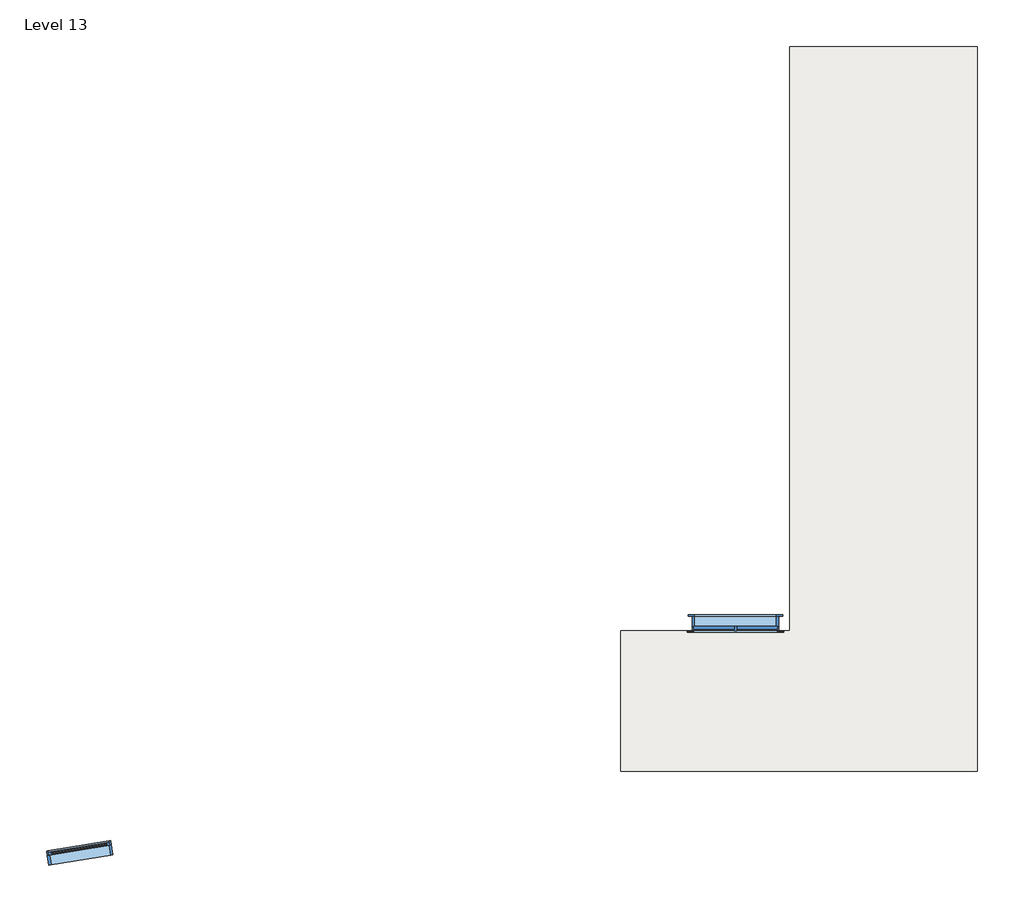
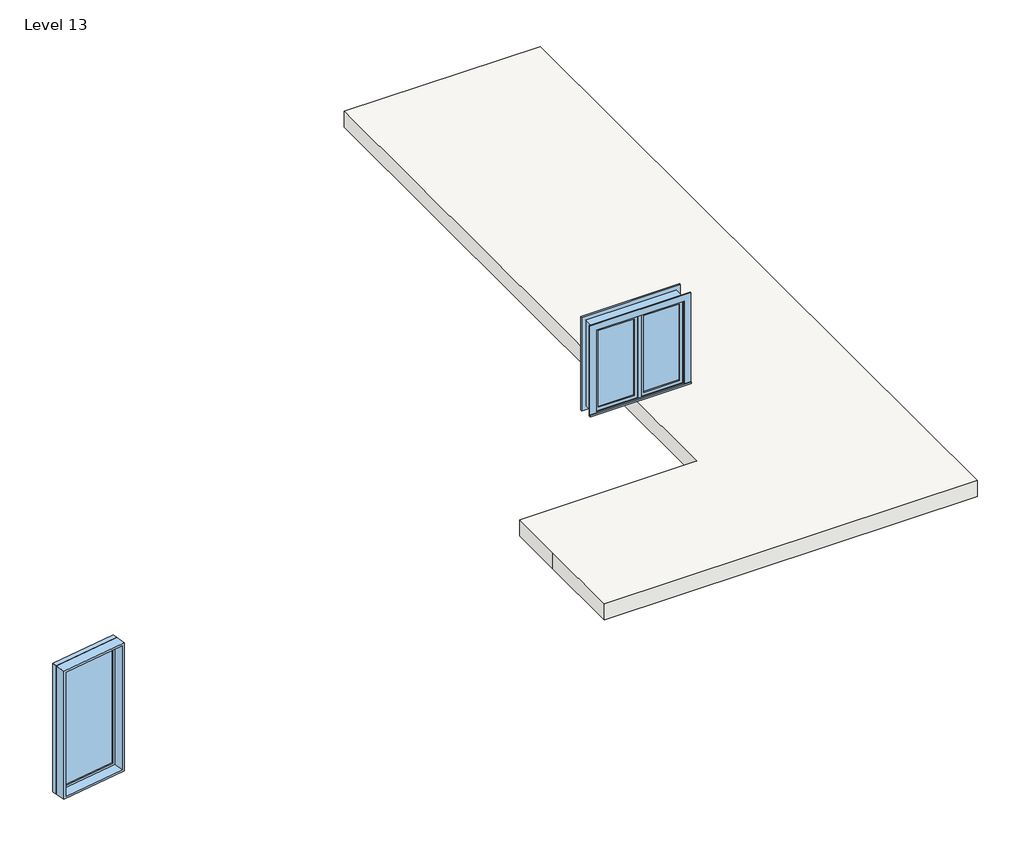
# One storey: 2 windows, 1 slab.
"""IFC4 building model written with IfcOpenShell, lengths in millimetres."""

from ifc_helpers import new_model, si_unit, frame, origin, place, context, project, spatial, polyline, outline, extrude, transform, mapped, element, save
from components import window_0862ab64, window_9a779fa2

model = new_model("IFC4")

# Units and contexts
model_context = context("Model", 3, world=origin())
ifc_project = project(units=[si_unit("LENGTHUNIT", "METRE", prefix="MILLI")], contexts=[model_context])

# Site, building, storey
site = spatial("IfcSite", under=ifc_project)
building = spatial("IfcBuilding", under=site)
storey = spatial("IfcBuildingStorey", under=building, Name="Level 13", Elevation=19659.6)

# Slab
placement = place(None, origin())
element("IfcSlab", 1, ObjectType="9\"", at=placement, inside=storey, context=model_context, shape_type="SweptSolid", body=[
    extrude(outline(polyline([(5039.2964723, -14840.0808221), (5039.2964723, -14078.0808221), (7223.6964723, -14078.0808221), (7426.8964723, -14078.0808221), (7426.8964723, -5848.4808221), (10068.4964723, -5848.4808221), (10068.4964723, -14840.0808221), (10068.4964723, -16059.2808221), (5039.2964723, -16059.2808221), (5039.2964723, -14840.0808221)])), frame((0.0, 0.0, 19431.0), z_axis=(0.0, 0.0, 1.0), x_axis=(1.0, 0.0, 0.0)), (0.0, 0.0, 1.0), 228.6),
])

# Windows
window_shape = window_0862ab64(model_context)
element("IfcWindow", 2, ObjectType="Casement Dbl with Trim : 48\" x 48\"", at=placement, inside=storey, context=model_context, shape_type="MappedRepresentation", body=[
    mapped(window_shape, transform((6658.4494573, -13957.4308221, 19899.9127534), x_axis=(-1.0, 0.0, 0.0), y_axis=(0.0, -1.0, 0.0), z_axis=(0.0, 0.0, 1.0))),
])
window_2_shape = window_9a779fa2(model_context)
element("IfcWindow", 3, ObjectType="Fixed : 36\" x 72\"", at=placement, inside=storey, context=model_context, shape_type="MappedRepresentation", body=[
    mapped(window_2_shape, transform((-2543.099786, -17204.6888165, 20190.5324703), x_axis=(0.9866375910039796, 0.16293024279692148, 0.0), y_axis=(-0.16293024279692148, 0.9866375910039796, 0.0), z_axis=(0.0, 0.0, 1.0))),
])

save(model, "model.ifc")

# Revit data of these elements
# Type "9\""
#   Assembly Code = "B1010"
#   Function = 0
#   Layers, outside or top first: 0' - 9" no material (function 1)
# Type "Casement Dbl with Trim : 48\" x 48\""
#   Type Mark = "10"
#   Construction Type Id = "GSP4R"
#   Assembly Code = "B2020100"
#   Analytic Construction = "1/8 in Pilkington single glazing"
#   Visual Light Transmittance = 0.9
#   Solar Heat Gain Coefficient = 0.78
#   Heat Transfer Coefficient (U) = 0.6496 BTU/(h·ft²·°F)
#   Height = 4' - 0"
#   Default Sill Height = 3' - 0"
#   Trim Projection - Ext. = 0' - 0 1/2"
#   Trim Projection - Int. = 0' - 0 3/4"
#   Trim Width - Exterior = 0' - 3 1/2"
#   Trim Width - Interior = 0' - 3 1/2"
#   Width = 4' - 0"
#   Window Inset = 0' - 0 3/4"
#   Define Thermal Properties by = 1
#   Glass Pane Material = Glass
#   Sash Material = Sash
#   Trim Exterior Material = Trim
#   Trim Interior Material = Trim
#   Wall Closure = (empty or 0)
# Type "Fixed : 36\" x 72\""
#   Type Mark = "9"
#   Construction Type Id = "GSP4R"
#   Assembly Code = "B2020100"
#   Analytic Construction = "1/8 in Pilkington single glazing"
#   Visual Light Transmittance = 0.9
#   Solar Heat Gain Coefficient = 0.78
#   Heat Transfer Coefficient (U) = 0.6496 BTU/(h·ft²·°F)
#   Height = 6' - 0"
#   Default Sill Height = 1' - 0"
#   Width = 3' - 0"
#   Window Inset = 0' - 0 3/4"
#   Define Thermal Properties by = 1
#   Glass Pane Material = Glass
#   Sash Material = Sash
#   Wall Closure = (empty or 0)
# Element 1 (IfcSlab, "9\"")
#   built-in parameter 1001955 = -1.5708 (stored number, unit not read)
#   Height Offset From Level = 0' - 0"
#   Phase Created = New Construction
#   Materials on its faces: "Default Floor"
# Element 2 (IfcWindow, "Casement Dbl with Trim : 48\" x 48\"")
#   Mark = "55"
#   Phase Created = New Construction
#   Materials on its faces: "Sash", "Trim", "Glass"
# Element 3 (IfcWindow, "Fixed : 36\" x 72\"")
#   Mark = "10"
#   Phase Created = New Construction
#   Materials on its faces: "Sash", "Glass"
# Materials
#   "Glass": class "Glass", colour RGB 0 128 192, transparency 0.75, Description = "Soda Lime Glass", Cost = 0
#   "Sash": class "Wood", colour RGB 224 178 126, transparency 0
#   "Trim": class "Wood", colour RGB 224 178 126, transparency 0
#   "Default Floor": colour RGB 128 128 128, transparency 0
